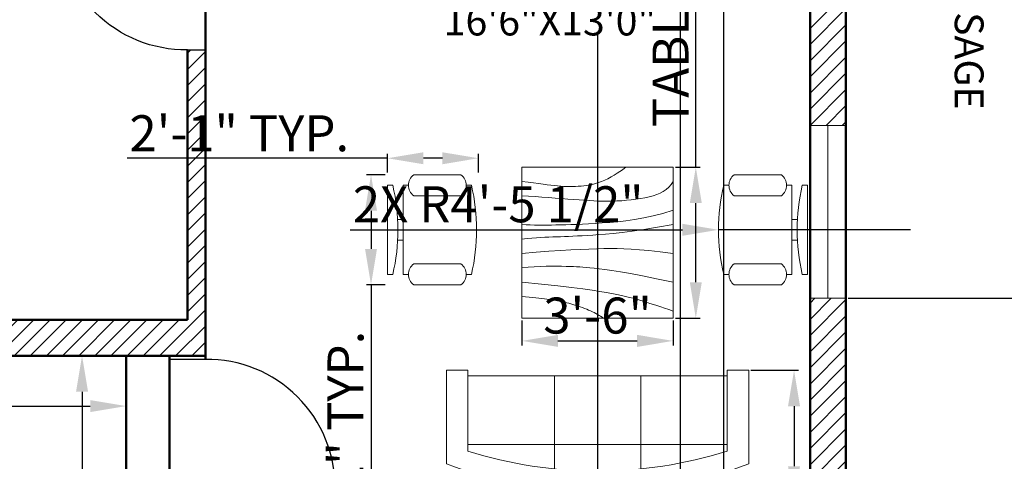
# Model space of a CAD drawing. Units: inches. Extents: x 2206 to 2843, y 1750 to 2489.
# Tile 3 of 8: x 2428 to 2702, y 1953 to 2075. Entities that reach past the tile are written whole.
import ezdxf

# ---------------------------------------------------------------- set-up
doc = ezdxf.new("R2010")
doc.units = ezdxf.units.IN
for name, color, linetype, lineweight in [('A-ANNO-DIMS', 2, 'Continuous', 18), ('A-AREA-IDEN', 7, 'Continuous', 18), ('A-DOOR', 3, 'Continuous', 25), ('A-FURN', 21, 'Continuous', 18), ('A-GLAZ', 4, 'Continuous', 18), ('A-WALL', 7, 'Continuous', 50), ('A-WALL-PATT', 252, 'Continuous', 13)]:
    doc.layers.add(name, color=color, linetype=linetype, lineweight=lineweight)
doc.styles.get("Standard").update_dxf_attribs({"font": 'arial.ttf'})
doc.dimstyles.new('ISO-25', dxfattribs={"dimtxt": 10, "dimasz": 10, "dimexe": 1.25, "dimexo": 0.625, "dimtad": 1, "dimdec": 1, "dimlunit": 3, "dimtxsty": 'Standard', "dimcen": 2.5, "dimadec": 0, "dimazin": 0, "dimtfac": 1, "dimtdec": 1, "dimtmove": 0, "dimatfit": 3, "dimfxl": 1, "dimarcsym": 0})

# ---------------------------------------------------------------- blocks, each defined once
blk = doc.blocks.new('Chair - Desk')
for p, q in [((-8.5, 0), (-8.5, -1)), ((-8.5, 0), (8.5, 0)), ((8.5, 0), (8.5, -1)), ((-8.5, -3), (-8.5, -4)), ((-8.5, -3), (8.5, -3)), ((-2, -3), (-2, -1.9355)), ((2, -1.9576), (2, -3)), ((8.5, -3), (8.5, -4)), ((-10.5, -5), (-10.5, -14)), ((-6.5, -14), (-6.5, -5)), ((6.5, -5), (6.5, -14)), ((10.5, -14), (10.5, -5)), ((-8.5, -15), (-8.5, -16)), ((8.5, -15), (8.5, -16))]:
    blk.add_line(p, q)
for centre, radius, start, end in [((0, 34.625), 36.625, 256.5803, 283.4197), ((-8.5, -6.5), 2.5, 36.8699, 143.1301), ((8.5, -6.5), 2.5, 36.8699, 143.1301), ((-8.5, -12.5), 2.5, 216.8699, 323.1301), ((8.5, -12.5), 2.5, 216.8699, 323.1301), ((0, 19.625), 36.625, 256.5803, 283.4197)]:
    blk.add_arc(centre, radius, start, end)
blk = doc.blocks.new('Table - Square Woodgrain 42 x 42 in.')
blk.add_line((0, -42), (42, -42))
for points in [[(0, -4), (1.704, -4.2172), (3.2358, -4.4188), (4.615, -4.604), (5.8615, -4.7721), (6.9951, -4.9224), (8.0357, -5.0541), (9.0031, -5.1667), (9.9171, -5.2594), (10.7951, -5.3316), (11.6445, -5.3836), (12.4702, -5.4157), (13.277, -5.4283), (14.0698, -5.4217), (14.8535, -5.3964), (15.6331, -5.3526), (16.4133, -5.2908), (17.1986, -5.2103), (17.9913, -5.1062), (18.793, -4.9727), (19.6056, -4.8038), (20.4307, -4.5937), (21.2701, -4.3365), (22.1256, -4.0262), (22.9989, -3.6571), (23.888, -3.2272), (24.7756, -2.7516), (25.6408, -2.2491), (26.4624, -1.7387), (27.2195, -1.2395), (27.891, -0.7703), (28.456, -0.3501), (28.8934, 0.002)], [(0, -42), (0, 0), (42, 0), (42, -42)], [(0, -8), (1.8203, -8.1001), (3.6741, -8.2149), (5.5411, -8.3408), (7.4011, -8.4741), (9.2339, -8.6112), (11.0193, -8.7484), (12.7371, -8.8821), (14.3671, -9.0086), (15.8954, -9.1246), (17.3337, -9.2278), (18.6997, -9.3159), (20.0116, -9.387), (21.2871, -9.4389), (22.5442, -9.4696), (23.8008, -9.477), (25.0749, -9.459), (26.3791, -9.4137), (27.7049, -9.3403), (29.0383, -9.2382), (30.3655, -9.1068), (31.6728, -8.9455), (32.9461, -8.7535), (34.1717, -8.5304), (35.3358, -8.2756), (36.4268, -7.9863), (37.443, -7.6521), (38.3849, -7.2603), (39.253, -6.7986), (40.048, -6.2542), (40.7705, -5.6147), (41.421, -4.8674), (42, -4)], [(42, -12), (39.1784, -12.8621), (36.4519, -13.5654), (33.8246, -14.1294), (31.3004, -14.5731), (28.8832, -14.9161), (26.577, -15.1775), (24.3858, -15.3768), (22.3136, -15.5332), (20.3622, -15.6632), (18.5254, -15.7718), (16.7947, -15.8612), (15.1618, -15.9338), (13.6183, -15.9916), (12.1558, -16.0369), (10.7659, -16.0718), (9.4403, -16.0987), (8.1703, -16.1191), (6.9461, -16.1325), (5.7577, -16.1377), (4.595, -16.1335), (3.4479, -16.1188), (2.3064, -16.0924), (1.1604, -16.0532), (0, -16)], [(42, -16), (37.6529, -16.7365), (33.8802, -17.329), (30.6179, -17.7961), (27.8015, -18.1561), (25.3668, -18.4275), (23.2497, -18.6288), (21.3859, -18.7785), (19.7111, -18.8949), (18.1693, -18.9939), (16.7375, -19.0795), (15.401, -19.1534), (14.1449, -19.217), (12.9544, -19.2717), (11.8148, -19.3191), (10.7113, -19.3606), (9.6291, -19.3976), (8.5534, -19.4323), (7.47, -19.4689), (6.3643, -19.5122), (5.222, -19.5672), (4.0288, -19.6386), (2.7703, -19.7313), (1.4321, -19.8501), (0, -20)], [(0, -24), (3.9243, -23.6805), (7.4766, -23.4138), (10.6891, -23.1954), (13.5943, -23.0205), (16.2247, -22.8847), (18.6125, -22.7832), (20.7903, -22.7116), (22.7903, -22.6651), (24.6563, -22.642), (26.4764, -22.6507), (28.35, -22.7024), (30.3766, -22.8084), (32.6555, -22.98), (35.2861, -23.2283), (38.3678, -23.5645), (42, -24)], [(42, -32), (37.392, -31.017), (33.4585, -30.2231), (30.1291, -29.5949), (27.3334, -29.109), (25.0009, -28.742), (23.0612, -28.4707), (21.4439, -28.2716), (20.0786, -28.1215), (18.8998, -28.0002), (17.8609, -27.9014), (16.9206, -27.8219), (16.0371, -27.7588), (15.1691, -27.709), (14.2748, -27.6693), (13.3128, -27.6368), (12.2415, -27.6083), (11.0295, -27.5824), (9.6867, -27.5643), (8.233, -27.5608), (6.6884, -27.5787), (5.0728, -27.6248), (3.4062, -27.7058), (1.7086, -27.8286), (0, -28)], [(0, -32), (5.4026, -32.5358), (9.9494, -33.019), (13.7424, -33.4553), (16.8834, -33.8505), (19.4743, -34.2106), (21.6171, -34.5413), (23.4136, -34.8486), (24.9657, -35.1382), (26.3614, -35.4156), (27.6332, -35.6841), (28.7995, -35.9467), (29.8788, -36.2064), (30.8897, -36.4661), (31.8507, -36.7288), (32.7802, -36.9973), (33.6968, -37.2747), (34.6175, -37.5635), (35.5531, -37.8651), (36.5128, -38.1805), (37.506, -38.5108), (38.5421, -38.8568), (39.6302, -39.2197), (40.7797, -39.6004), (42, -40)], [(0, -36), (3.0098, -36.2857), (5.5354, -36.5643), (7.6368, -36.8359), (9.374, -37.1009), (10.807, -37.3597), (11.9957, -37.6126), (13.0002, -37.8599), (13.8804, -38.102), (14.6874, -38.3393), (15.4365, -38.5729), (16.1338, -38.8041), (16.7858, -39.0341), (17.3987, -39.264), (17.9787, -39.4952), (18.5322, -39.7288), (19.0655, -39.9662), (19.5832, -40.2081), (20.0842, -40.4544), (20.5657, -40.7046), (21.0249, -40.9581), (21.459, -41.2144), (21.8653, -41.4731), (22.2409, -41.7335), (22.5831, -41.9951)]]:
    blk.add_lwpolyline(points)
blk = doc.blocks.new('Sofa - Roundback 7 ft.')
for p, q in [((-12.00002, -32.4421), (-12.00003, -6.5971)), ((11.99997, -32.4421), (11.99998, -6.5971)), ((-36.000027, -34), (-36.000027, -11.4696)), ((-35.999844, -13.3819), (35.9998, -13.3819)), ((35.99998, -34), (35.99998, -11.4696)), ((-36.000027, -32.4421), (35.99998, -32.4421))]:
    blk.add_line(p, q)
for points in [[(-36.000027, -34), (-42.000027, -34), (-42.000027, -8)], [(41.99998, -8), (41.99998, -34), (35.99998, -34)]]:
    blk.add_lwpolyline(points)
for centre, radius, start, end in [((0, -114.25), 114.25, 68.43141, 111.5686), ((-0.00001, -127.1968), 121.1968, 72.72033, 107.2797)]:
    blk.add_arc(centre, radius, start, end)
blk = doc.blocks.new('*D17')
at = {"layer": 'A-ANNO-DIMS', "color": 0, "lineweight": -2, "transparency": 16777216}
for p, q in [((2296.58, 1981.27), (2296.58, 1966.68)), ((2457.58, 1981.27), (2457.58, 1966.68)), ((2306.58, 1967.93), (2447.58, 1967.93))]:
    blk.add_line(p, q, dxfattribs=at)
at = {"layer": 'A-ANNO-DIMS', "color": 0, "transparency": 16777216}
for points in [[(2306.58, 1969.6), (2306.58, 1966.26), (2296.58, 1967.93)], [(2447.58, 1969.6), (2447.58, 1966.26), (2457.58, 1967.93)]]:
    blk.add_solid(points, dxfattribs=at)
at = {"layer": 'Defpoints', "color": 0, "transparency": 16777216}
for p in [(2296.58, 1981.9), (2457.58, 1981.9), (2457.58, 1967.93)]:
    blk.add_point(p, dxfattribs=at)
at = {"layer": 'A-ANNO-DIMS', "color": 0, "transparency": 16777216, "insert": (2377.08, 1973.66), "char_height": 10, "attachment_point": 5}
blk.add_mtext('13\'-5"', dxfattribs=at)
blk = doc.blocks.new('*D18')
at = {"layer": 'A-ANNO-DIMS', "color": 0, "lineweight": -2, "transparency": 16777216}
for p, q in [((2445.95, 1981.9), (2446.57, 1981.9)), ((2445.32, 1971.9), (2445.32, 1809.9)), ((2445.95, 1799.9), (2446.57, 1799.9))]:
    blk.add_line(p, q, dxfattribs=at)
at = {"layer": 'A-ANNO-DIMS', "color": 0, "transparency": 16777216}
for points in [[(2443.65, 1971.9), (2446.99, 1971.9), (2445.32, 1981.9)], [(2443.65, 1809.9), (2446.99, 1809.9), (2445.32, 1799.9)]]:
    blk.add_solid(points, dxfattribs=at)
at = {"layer": 'Defpoints', "color": 0, "transparency": 16777216}
for p in [(2445.32, 1981.9), (2445.32, 1799.9), (2445.32, 1799.9)]:
    blk.add_point(p, dxfattribs=at)
at = {"layer": 'A-ANNO-DIMS', "color": 0, "transparency": 16777216, "insert": (2439.59, 1890.9), "char_height": 10, "attachment_point": 5, "rotation": 90}
blk.add_mtext('15\'-2"', dxfattribs=at)
blk = doc.blocks.new('WIN-48IN')
for p, q in [((0, 10), (0, 0)), ((48, 10), (48, 0)), ((48, 5), (0, 5))]:
    blk.add_line(p, q)
blk = doc.blocks.new('DOOR-SWING-36IN')
for p, q in [((0, 5), (0, 41)), ((1, 0), (1, 41)), ((0, 5), (0, 0)), ((36, 5), (36, 0))]:
    blk.add_line(p, q)
blk.add_arc((0.5, 5.5), 35.5, 359.1931, 90.8069)
blk = doc.blocks.new('*D45')
at = {"layer": 'A-ANNO-DIMS', "color": 0, "lineweight": -2, "transparency": 16777216}
for p, q in [((2529.57, 2032.2), (2524.36, 2032.2)), ((2525.61, 2022.2), (2525.61, 2011.61)), ((2529.57, 2001.61), (2524.36, 2001.61)), ((2525.61, 2001.61), (2525.61, 1858.87))]:
    blk.add_line(p, q, dxfattribs=at)
at = {"layer": 'A-ANNO-DIMS', "color": 0, "transparency": 16777216}
for points in [[(2523.94, 2022.2), (2527.27, 2022.2), (2525.61, 2032.2)], [(2523.94, 2011.61), (2527.27, 2011.61), (2525.61, 2001.61)]]:
    blk.add_solid(points, dxfattribs=at)
at = {"layer": 'Defpoints', "color": 0, "transparency": 16777216}
for p in [(2530.19, 2032.2), (2525.61, 2001.61), (2530.19, 2001.61)]:
    blk.add_point(p, dxfattribs=at)
at = {"layer": 'A-ANNO-DIMS', "color": 0, "transparency": 16777216, "insert": (2519.81, 1925.24), "char_height": 10, "attachment_point": 5, "rotation": 90}
blk.add_mtext('CHAIR 2\'-6 1/2" TYP.', dxfattribs=at)
blk = doc.blocks.new('*D46')
at = {"layer": 'A-ANNO-DIMS', "color": 0, "lineweight": -2, "transparency": 16777216}
for p, q in [((2530.19, 2036.79), (2457.82, 2036.79)), ((2530.19, 2032.82), (2530.19, 2038.04)), ((2545.44, 2036.79), (2540.19, 2036.79)), ((2555.44, 2032.82), (2555.44, 2038.04))]:
    blk.add_line(p, q, dxfattribs=at)
at = {"layer": 'A-ANNO-DIMS', "color": 0, "transparency": 16777216}
for points in [[(2540.19, 2038.45), (2540.19, 2035.12), (2530.19, 2036.79)], [(2545.44, 2038.45), (2545.44, 2035.12), (2555.44, 2036.79)]]:
    blk.add_solid(points, dxfattribs=at)
at = {"layer": 'Defpoints', "color": 0, "transparency": 16777216}
for p in [(2530.19, 2036.79), (2530.19, 2032.2), (2555.44, 2032.2)]:
    blk.add_point(p, dxfattribs=at)
at = {"layer": 'A-ANNO-DIMS', "color": 0, "transparency": 16777216, "insert": (2489.01, 2042.44), "char_height": 10, "attachment_point": 5}
blk.add_mtext('2\'-1" TYP.', dxfattribs=at)
blk = doc.blocks.new('*D49')
at = {"layer": 'A-ANNO-DIMS', "color": 0, "lineweight": -2, "transparency": 16777216}
for p, q in [((2615.85, 2034.34), (2615.85, 2120.57)), ((2610.18, 2034.34), (2617.1, 2034.34)), ((2615.85, 2002.34), (2615.85, 2024.34)), ((2610.18, 1992.34), (2617.1, 1992.34))]:
    blk.add_line(p, q, dxfattribs=at)
at = {"layer": 'A-ANNO-DIMS', "color": 0, "transparency": 16777216}
for points in [[(2614.19, 2024.34), (2617.52, 2024.34), (2615.85, 2034.34)], [(2614.19, 2002.34), (2617.52, 2002.34), (2615.85, 1992.34)]]:
    blk.add_solid(points, dxfattribs=at)
at = {"layer": 'Defpoints', "color": 0, "transparency": 16777216}
for p in [(2609.55, 2034.34), (2615.85, 2034.34), (2609.55, 1992.34)]:
    blk.add_point(p, dxfattribs=at)
at = {"layer": 'A-ANNO-DIMS', "color": 0, "transparency": 16777216, "insert": (2610.12, 2082.46), "char_height": 10, "attachment_point": 5, "rotation": 90}
blk.add_mtext('TABLE 3\'-6"', dxfattribs=at)
blk = doc.blocks.new('*D50')
at = {"layer": 'A-ANNO-DIMS', "color": 0, "lineweight": -2, "transparency": 16777216}
for p, q in [((2567.55, 1991.72), (2567.55, 1984.79)), ((2609.55, 1991.72), (2609.55, 1984.79)), ((2577.55, 1986.04), (2599.55, 1986.04))]:
    blk.add_line(p, q, dxfattribs=at)
at = {"layer": 'A-ANNO-DIMS', "color": 0, "transparency": 16777216}
for points in [[(2577.55, 1987.71), (2577.55, 1984.37), (2567.55, 1986.04)], [(2599.55, 1987.71), (2599.55, 1984.37), (2609.55, 1986.04)]]:
    blk.add_solid(points, dxfattribs=at)
at = {"layer": 'Defpoints', "color": 0, "transparency": 16777216}
for p in [(2567.55, 1992.34), (2609.55, 1992.34), (2609.55, 1986.04)]:
    blk.add_point(p, dxfattribs=at)
at = {"layer": 'A-ANNO-DIMS', "color": 0, "transparency": 16777216, "insert": (2588.55, 1991.78), "char_height": 10, "attachment_point": 5}
blk.add_mtext('3\'-6"', dxfattribs=at)
blk = doc.blocks.new('*D52')
at = {"layer": 'A-ANNO-DIMS', "color": 0, "lineweight": -2, "transparency": 16777216}
for p, q in [((2631.17, 1977.9), (2644.4, 1977.9)), ((2643.15, 1967.9), (2643.15, 1951.23)), ((2631.17, 1941.23), (2644.4, 1941.23)), ((2643.15, 1941.23), (2643.15, 1880.11))]:
    blk.add_line(p, q, dxfattribs=at)
at = {"layer": 'A-ANNO-DIMS', "color": 0, "transparency": 16777216}
for points in [[(2641.48, 1967.9), (2644.81, 1967.9), (2643.15, 1977.9)], [(2641.48, 1951.23), (2644.81, 1951.23), (2643.15, 1941.23)]]:
    blk.add_solid(points, dxfattribs=at)
at = {"layer": 'Defpoints', "color": 0, "transparency": 16777216}
for p in [(2630.55, 1977.9), (2630.55, 1941.23), (2643.15, 1941.23)]:
    blk.add_point(p, dxfattribs=at)
at = {"layer": 'A-ANNO-DIMS', "color": 0, "transparency": 16777216, "insert": (2637.35, 1905.67), "char_height": 10, "attachment_point": 5, "rotation": 90}
blk.add_mtext('3\'-0 1/2"', dxfattribs=at)
blk = doc.blocks.new('*D63')
at = {"layer": 'A-ANNO-DIMS', "color": 0, "lineweight": -2, "transparency": 16777216}
for p, q in [((2647.58, 2246.27), (2647.58, 1757.6)), ((2657.58, 2246.27), (2657.58, 1757.6)), ((2637.58, 1758.85), (2627.58, 1758.85)), ((2647.58, 1758.85), (2657.58, 1758.85)), ((2667.58, 1758.85), (2713.18, 1758.85))]:
    blk.add_line(p, q, dxfattribs=at)
at = {"layer": 'A-ANNO-DIMS', "color": 0, "transparency": 16777216}
for points in [[(2637.58, 1760.52), (2637.58, 1757.18), (2647.58, 1758.85)], [(2667.58, 1760.52), (2667.58, 1757.18), (2657.58, 1758.85)]]:
    blk.add_solid(points, dxfattribs=at)
at = {"layer": 'Defpoints', "color": 0, "transparency": 16777216}
for p in [(2647.58, 2246.9), (2657.58, 2246.9), (2657.58, 1758.85)]:
    blk.add_point(p, dxfattribs=at)
at = {"layer": 'A-ANNO-DIMS', "color": 0, "transparency": 16777216, "insert": (2695.38, 1764.58), "char_height": 10, "attachment_point": 5}
blk.add_mtext('0\'-10"', dxfattribs=at)
blk = doc.blocks.new('*D69')
at = {"layer": 'A-ANNO-DIMS', "color": 0, "lineweight": -2, "transparency": 16777216}
for p, q in [((2658.2, 1997.9), (2747.88, 1997.9)), ((2746.63, 1987.9), (2746.63, 1943.9)), ((2648.2, 1933.9), (2747.88, 1933.9))]:
    blk.add_line(p, q, dxfattribs=at)
at = {"layer": 'A-ANNO-DIMS', "color": 0, "transparency": 16777216}
for points in [[(2744.96, 1987.9), (2748.3, 1987.9), (2746.63, 1997.9)], [(2744.96, 1943.9), (2748.3, 1943.9), (2746.63, 1933.9)]]:
    blk.add_solid(points, dxfattribs=at)
at = {"layer": 'Defpoints', "color": 0, "transparency": 16777216}
for p in [(2657.58, 1997.9), (2647.58, 1933.9), (2746.63, 1933.9)]:
    blk.add_point(p, dxfattribs=at)
at = {"layer": 'A-ANNO-DIMS', "color": 0, "transparency": 16777216, "insert": (2740.92, 1965.9), "char_height": 10, "attachment_point": 5, "rotation": 90}
blk.add_mtext('5\'-4"', dxfattribs=at)
blk = doc.blocks.new('*D71')
at = {"layer": 'A-ANNO-DIMS', "color": 0, "lineweight": -2, "transparency": 16777216}
for p, q in [((2218.53, 1943.9), (2218.53, 1980.79)), ((2646.95, 1933.9), (2217.28, 1933.9)), ((2218.53, 1918.9), (2218.53, 1933.9)), ((2656.95, 1918.9), (2217.28, 1918.9)), ((2218.53, 1908.9), (2218.53, 1898.9))]:
    blk.add_line(p, q, dxfattribs=at)
at = {"layer": 'A-ANNO-DIMS', "color": 0, "transparency": 16777216}
for points in [[(2216.86, 1943.9), (2220.2, 1943.9), (2218.53, 1933.9)], [(2216.86, 1908.9), (2220.2, 1908.9), (2218.53, 1918.9)]]:
    blk.add_solid(points, dxfattribs=at)
at = {"layer": 'Defpoints', "color": 0, "transparency": 16777216}
for p in [(2218.53, 1933.9), (2647.58, 1933.9), (2657.58, 1918.9)]:
    blk.add_point(p, dxfattribs=at)
at = {"layer": 'A-ANNO-DIMS', "color": 0, "transparency": 16777216, "insert": (2212.8, 1967.34), "char_height": 10, "attachment_point": 5, "rotation": 90}
blk.add_mtext('1\'-3"', dxfattribs=at)
blk = doc.blocks.new('*D74')
at = {"layer": 'A-ANNO-DIMS', "color": 0, "lineweight": -2, "transparency": 16777216}
for p, q in [((2611.58, 1856.52), (2611.58, 2432.2)), ((2647.58, 1856.52), (2647.58, 2432.2)), ((2621.58, 2430.95), (2637.58, 2430.95))]:
    blk.add_line(p, q, dxfattribs=at)
at = {"layer": 'A-ANNO-DIMS', "color": 0, "transparency": 16777216}
for points in [[(2621.58, 2432.62), (2621.58, 2429.28), (2611.58, 2430.95)], [(2637.58, 2432.62), (2637.58, 2429.28), (2647.58, 2430.95)]]:
    blk.add_solid(points, dxfattribs=at)
at = {"layer": 'Defpoints', "color": 0, "transparency": 16777216}
for p in [(2647.58, 2430.95), (2611.58, 1855.9), (2647.58, 1855.9)]:
    blk.add_point(p, dxfattribs=at)
at = {"layer": 'A-ANNO-DIMS', "color": 0, "transparency": 16777216, "insert": (2629.58, 2436.68), "char_height": 10, "attachment_point": 5}
blk.add_mtext('3\'-0"', dxfattribs=at)
blk = doc.blocks.new('*D77')
at = {"layer": 'A-ANNO-DIMS', "color": 0, "lineweight": -2, "transparency": 16777216}
for p, q in [((2623.58, 2204.27), (2623.58, 1757.6)), ((2647.58, 2204.27), (2647.58, 1757.6)), ((2633.58, 1758.85), (2637.58, 1758.85)), ((2647.58, 1758.85), (2685.58, 1758.85))]:
    blk.add_line(p, q, dxfattribs=at)
at = {"layer": 'A-ANNO-DIMS', "color": 0, "transparency": 16777216}
for points in [[(2633.58, 1760.52), (2633.58, 1757.18), (2623.58, 1758.85)], [(2637.58, 1760.52), (2637.58, 1757.18), (2647.58, 1758.85)]]:
    blk.add_solid(points, dxfattribs=at)
at = {"layer": 'Defpoints', "color": 0, "transparency": 16777216}
for p in [(2623.58, 2204.9), (2647.58, 2204.9), (2647.58, 1758.85)]:
    blk.add_point(p, dxfattribs=at)
at = {"layer": 'A-ANNO-DIMS', "color": 0, "transparency": 16777216, "insert": (2671.58, 1764.58), "char_height": 10, "attachment_point": 5}
blk.add_mtext('2\'-0"', dxfattribs=at)
blk = doc.blocks.new('*D80')
at = {"layer": 'A-ANNO-DIMS', "color": 0, "lineweight": -2, "transparency": 16777216}
for p, q in [((2588.55, 2071.1), (2588.55, 1949.9)), ((2588.55, 1854.6), (2588.55, 1939.9))]:
    blk.add_line(p, q, dxfattribs=at)
at = {"layer": 'A-ANNO-DIMS', "color": 0, "transparency": 16777216}
blk.add_solid([(2590.21, 1939.9), (2586.88, 1939.9), (2588.55, 1949.9)], dxfattribs=at)
at = {"layer": 'Defpoints', "color": 0, "transparency": 16777216}
for p in [(2588.55, 2071.1), (2588.55, 1949.9)]:
    blk.add_point(p, dxfattribs=at)
at = {"layer": 'A-ANNO-DIMS', "color": 0, "transparency": 16777216, "insert": (2594.28, 1877.18), "char_height": 10, "attachment_point": 5, "rotation": 270.0002}
blk.add_mtext('R10\'-1"', dxfattribs=at)
blk = doc.blocks.new('*D81')
at = {"layer": 'A-ANNO-DIMS', "color": 0, "lineweight": -2, "transparency": 16777216}
for p, q in [((2588.55, 2058.15), (2588.55, 1943.9)), ((2588.55, 1845), (2588.55, 1933.9))]:
    blk.add_line(p, q, dxfattribs=at)
at = {"layer": 'A-ANNO-DIMS', "color": 0, "transparency": 16777216}
blk.add_solid([(2590.21, 1933.9), (2586.88, 1933.9), (2588.55, 1943.9)], dxfattribs=at)
at = {"layer": 'Defpoints', "color": 0, "transparency": 16777216}
for p in [(2588.55, 2058.15), (2588.55, 1943.9)]:
    blk.add_point(p, dxfattribs=at)
at = {"layer": 'A-ANNO-DIMS', "color": 0, "transparency": 16777216, "insert": (2594.34, 1875.35), "char_height": 10, "attachment_point": 5, "rotation": 270.0002}
blk.add_mtext('R9\'-6 1/2"', dxfattribs=at)
blk = doc.blocks.new('*D82')
at = {"layer": 'A-ANNO-DIMS', "color": 0, "lineweight": -2, "transparency": 16777216}
for p, q in [((2519.78, 2016.9), (2612.14, 2016.9)), ((2675.49, 2016.9), (2622.14, 2016.9))]:
    blk.add_line(p, q, dxfattribs=at)
at = {"layer": 'A-ANNO-DIMS', "color": 0, "transparency": 16777216}
blk.add_solid([(2612.14, 2018.57), (2612.14, 2015.24), (2622.14, 2016.9)], dxfattribs=at)
at = {"layer": 'Defpoints', "color": 0, "transparency": 16777216}
for p in [(2622.14, 2016.9), (2675.49, 2016.9)]:
    blk.add_point(p, dxfattribs=at)
at = {"layer": 'A-ANNO-DIMS', "color": 0, "transparency": 16777216, "insert": (2560.96, 2022.7), "char_height": 10, "attachment_point": 5, "rotation": 0.0005}
blk.add_mtext('2X R4\'-5 1/2"', dxfattribs=at)

msp = doc.modelspace()

# ---------------------------------------------------------------- hatches: boundary and pattern name
at = {"layer": 'A-WALL-PATT'}
h = msp.add_hatch(dxfattribs=at)
h.set_pattern_fill('ANSI31', color=256)
h.paths.add_polyline_path([(2710.58, 2394.9), (2296.58, 2394.9), (2296.58, 2335.9), (2306.58, 2335.9), (2306.58, 2384.9), (2479.58, 2384.9), (2652.58, 2384.9), (2700.58, 2384.9), (2700.58, 2300.9), (2690.58, 2300.9), (2690.58, 2290.9), (2710.58, 2290.9)])
h.paths.add_polyline_path([(2306.58, 2295.9), (2296.58, 2295.9), (2296.58, 2225.9), (2306.58, 2225.9), (2306.58, 2241.9)])
h.paths.add_polyline_path([(2306.58, 2111.9), (2306.58, 2132.9), (2296.58, 2132.9), (2296.58, 2071.9), (2306.58, 2071.9)])
h.paths.add_polyline_path([(2306.58, 2197.9), (2296.58, 2197.9), (2296.58, 2160.9), (2306.58, 2160.9), (2306.58, 2176.9)])
h.paths.add_polyline_path([(2370.58, 1991.9), (2306.58, 1991.9), (2306.58, 2031.9), (2296.58, 2031.9), (2296.58, 1981.9), (2370.58, 1981.9)])
h.paths.add_polyline_path([(2479.58, 2066.9), (2474.58, 2066.9), (2474.58, 1991.9), (2410.58, 1991.9), (2410.58, 1981.9), (2479.58, 1981.9)])
h.paths.add_polyline_path([(2539.58, 1943.9), (2479.58, 1943.9), (2479.58, 1944.9), (2469.58, 1944.9), (2469.58, 1933.9), (2539.58, 1933.9)])
h.paths.add_polyline_path([(2657.58, 1997.9), (2647.58, 1997.9), (2647.58, 1943.9), (2647.58, 1918.9), (2657.58, 1918.9)])
h.paths.add_polyline_path([(2647.58, 1943.9), (2587.58, 1943.9), (2587.58, 1933.9), (2647.58, 1933.9)])
h.paths.add_polyline_path([(2657.58, 2158.4), (2647.58, 2158.4), (2647.58, 2104.9), (2647.58, 2045.9), (2657.58, 2045.9)])
h.paths.add_polyline_path([(2657.58, 2204.89), (2647.58, 2204.89), (2647.58, 2188.4), (2657.58, 2188.4)])
h.paths.add_polyline_path([(2657.58, 2246.9), (2647.58, 2246.9), (2647.58, 2234.9), (2657.58, 2234.9)])
h.paths.add_polyline_path([(2662.58, 2300.9), (2652.58, 2300.9), (2652.58, 2346.22), (2647.58, 2346.22), (2647.58, 2290.9), (2662.58, 2290.9)])
h.paths.add_polyline_path([(2647.58, 2246.9), (2524.58, 2246.9), (2524.58, 2241.9), (2647.58, 2241.9)])
h.paths.add_polyline_path([(2351.58, 2246.9), (2306.58, 2246.9), (2306.58, 2241.9), (2351.58, 2241.9)])
h.paths.add_polyline_path([(2429.58, 2246.9), (2381.58, 2246.9), (2381.58, 2241.9), (2390.58, 2241.9), (2390.58, 2181.9), (2306.58, 2181.9), (2306.58, 2176.9), (2390.58, 2176.9), (2390.58, 2116.9), (2381.58, 2116.9), (2381.58, 2111.9), (2474.58, 2111.9), (2474.58, 2102.9), (2479.58, 2102.9), (2479.58, 2104.9), (2479.58, 2116.9), (2395.58, 2116.9), (2395.58, 2176.9), (2395.58, 2241.9), (2429.58, 2241.9)])
h.paths.add_polyline_path([(2479.58, 2384.9), (2474.58, 2384.9), (2474.58, 2246.9), (2465.58, 2246.9), (2465.58, 2241.9), (2479.58, 2241.9), (2488.58, 2241.9), (2488.58, 2246.9), (2479.58, 2246.9)])
h.paths.add_polyline_path([(2657.58, 1870.9), (2647.58, 1870.9), (2647.58, 1855.9), (2511.58, 1855.9), (2511.58, 1845.9), (2657.58, 1845.9)])

# ---------------------------------------------------------------- linework, layer by layer
at = {"layer": 'A-DOOR'}
msp.add_line((2479.58, 1980.9), (2469.58, 1980.9), dxfattribs=at)
msp.add_arc((2480.08, 1945.4), 35.5, 359.1931, 90.8069, dxfattribs=at)
at = {"layer": 'A-WALL'}
for p, q in [((2657.58, 2290.9), (2657.58, 1845.9)), ((2647.58, 2104.9), (2647.58, 1943.9)), ((2479.58, 2099.9), (2479.58, 1981.9)), ((2474.58, 1991.9), (2474.58, 2066.9)), ((2306.58, 1991.9), (2474.58, 1991.9)), ((2296.58, 1981.9), (2479.58, 1981.9)), ((2457.58, 1933.9), (2457.58, 1981.9)), ((2469.58, 1933.9), (2469.58, 1981.9)), ((2479.58, 1980.9), (2479.58, 1981.9))]:
    msp.add_line(p, q, dxfattribs=at)

# ---------------------------------------------------------------- block references
at = {"layer": 'A-DOOR', "extrusion": (0, 0, -1), "zscale": -1, "rotation": 270.0000000000001}
msp.add_blockref('DOOR-SWING-36IN', (-2479.58, 2102.9), dxfattribs=at)
at = {"layer": 'A-FURN'}
msp.add_blockref('Table - Square Woodgrain 42 x 42 in.', (2567.55, 2034.34), dxfattribs=at)
at = {"layer": 'A-FURN', "yscale": 1.456665205508952, "zscale": 1.456665205508952}
for p, xscale, rotation in [((2530.19, 2016.9), -1.456665205508952, 90), ((2646.9, 2016.9), 1.456665205508952, 270)]:
    msp.add_blockref('Chair - Desk', p, dxfattribs=dict(at, xscale=xscale, rotation=rotation))
at = {"layer": 'A-FURN', "rotation": 180}
msp.add_blockref('Sofa - Roundback 7 ft.', (2588.55, 1943.9), dxfattribs=at)
at = {"layer": 'A-GLAZ', "rotation": 270.0000000000006}
msp.add_blockref('WIN-48IN', (2647.58, 2045.9), dxfattribs=at)

# ---------------------------------------------------------------- texts
at = {"layer": 'A-AREA-IDEN', "insert": (2695.8, 2097.44), "char_height": 8, "attachment_point": 1, "rotation": 270}
msp.add_mtext_dynamic_manual_height_columns('PASSAGE', width=73.3542, gutter_width=12.5, heights=[0], dxfattribs=at)
at = {"layer": 'A-AREA-IDEN', "insert": (2529.31, 2092.24), "char_height": 8, "attachment_point": 1}
msp.add_mtext_dynamic_manual_height_columns('\\pxqc;DRAWING HALL\\P16\'6"X13\'0"', width=91.9993, gutter_width=12.5, heights=[0], dxfattribs=at)

# ---------------------------------------------------------------- dimensions: what is measured, and where the dimension line sits
at = {"layer": 'A-ANNO-DIMS'}
for base, p1, p2, override, picture, middle in [((2647.58, 2430.95), (2611.58, 1855.9), (2647.58, 1855.9), {"dimdec": 1, "dimlfac": 1, "dimrnd": 0, "dimzin": 1, "dimdsep": 46, "dimlunit": 4, "dimfrac": 2}, '*D74', (2629.58, 2436.68)), ((2657.58, 1758.85), (2647.58, 2246.9), (2657.58, 2246.9), {"dimdec": 1, "dimlfac": 1, "dimrnd": 0, "dimzin": 1, "dimdsep": 46, "dimlunit": 4, "dimfrac": 2}, '*D63', (2695.38, 1764.58)), ((2647.58, 1758.85), (2623.58, 2204.9), (2647.58, 2204.9), {"dimdec": 1, "dimlfac": 1, "dimrnd": 0, "dimzin": 1, "dimdsep": 46, "dimlunit": 4, "dimfrac": 2}, '*D77', (2671.58, 1764.58)), ((2609.55, 1986.04), (2567.55, 1992.34), (2609.55, 1992.34), {"dimdec": 1, "dimlfac": 1, "dimrnd": 0, "dimzin": 1, "dimdsep": 46, "dimlunit": 4, "dimfrac": 2}, '*D50', (2588.55, 1991.78)), ((2457.58, 1967.93), (2296.58, 1981.9), (2457.58, 1981.9), {"dimclrd": 0, "dimclre": 0, "dimclrt": 0}, '*D17', (2377.08, 1973.66))]:
    dim = msp.add_linear_dim(base=base, p1=p1, p2=p2, dimstyle='ISO-25', override=override, dxfattribs=at)
    dim.commit()
    dim.dimension.update_dxf_attribs({"geometry": picture, "text_midpoint": middle})
for base, p1, p2, angle, text, picture, middle in [((2615.85, 2034.34), (2609.55, 1992.34), (2609.55, 2034.34), 90, 'TABLE <>', '*D49', (2610.12, 2082.46)), ((2530.1942, 2036.7879), (2555.4431, 2032.1995), (2530.1942, 2032.1995), 180, '<> TYP.', '*D46', (2489.0064, 2042.4368)), ((2525.61, 2001.61), (2530.19, 2032.2), (2530.19, 2001.61), 270, 'CHAIR <> TYP.', '*D45', (2519.81, 1925.24))]:
    dim = msp.add_linear_dim(base=base, p1=p1, p2=p2, angle=angle, text=text, dimstyle='ISO-25', override={"dimdec": 1, "dimlfac": 1, "dimrnd": 0, "dimzin": 1, "dimdsep": 46, "dimlunit": 4, "dimfrac": 2}, dxfattribs=at)
    dim.commit()
    dim.dimension.update_dxf_attribs({"geometry": picture, "text_midpoint": middle})
for center, mpoint, picture, middle in [((2588.55, 2071.1), (2588.55, 1949.9), '*D80', (2588.55, 1877.18)), ((2588.547664, 2058.149218), (2588.548, 1943.899218), '*D81', (2588.5482016, 1875.349218))]:
    dim = msp.add_radius_dim(center=center, mpoint=mpoint, dimstyle='ISO-25', override={"dimdec": 1, "dimlfac": 1, "dimrnd": 0, "dimzin": 1, "dimdsep": 46, "dimlunit": 4, "dimfrac": 2}, dxfattribs=at)
    dim.commit()
    dim.dimension.update_dxf_attribs({"geometry": picture, "text_midpoint": middle, "dimtype": 164})
dim = msp.add_radius_dim(center=(2675.4882, 2016.9045), mpoint=(2622.1379, 2016.904), text='2X <>', dimstyle='ISO-25', override={"dimdec": 1, "dimlfac": 1, "dimrnd": 0, "dimzin": 1, "dimdsep": 46, "dimlunit": 4, "dimfrac": 2}, dxfattribs=at)
dim.commit()
dim.dimension.update_dxf_attribs({"geometry": '*D82', "text_midpoint": (2560.9569, 2022.699)})
for base, p1, p2, angle, override, picture, middle in [((2746.63, 1933.9), (2657.58, 1997.9), (2647.58, 1933.9), 90, {"dimdec": 1, "dimlfac": 1, "dimrnd": 0, "dimzin": 1, "dimdsep": 46, "dimlunit": 4, "dimfrac": 2}, '*D69', (2740.92, 1965.9)), ((2218.53, 1933.9), (2657.58, 1918.9), (2647.58, 1933.9), 90, {"dimdec": 1, "dimlfac": 1, "dimrnd": 0, "dimzin": 1, "dimdsep": 46, "dimlunit": 4, "dimfrac": 2}, '*D71', (2212.8, 1967.34)), ((2445.32, 1799.9), (2445.32, 1981.9), (2445.32, 1799.9), 90, {"dimclrd": 0, "dimclre": 0, "dimclrt": 0}, '*D18', (2439.59, 1890.9)), ((2643.15, 1941.23), (2630.55, 1977.9), (2630.55, 1941.23), 270, {"dimdec": 1, "dimlfac": 1, "dimrnd": 0, "dimzin": 1, "dimdsep": 46, "dimlunit": 4, "dimfrac": 2}, '*D52', (2637.35, 1905.67))]:
    dim = msp.add_linear_dim(base=base, p1=p1, p2=p2, angle=angle, dimstyle='ISO-25', override=override, dxfattribs=at)
    dim.commit()
    dim.dimension.update_dxf_attribs({"geometry": picture, "text_midpoint": middle})

doc.saveas('drawing.dxf')
